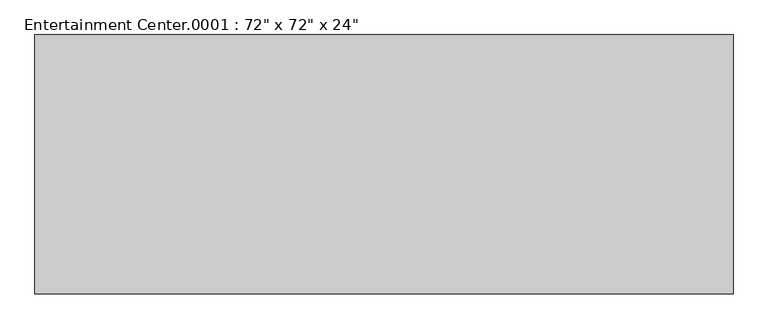
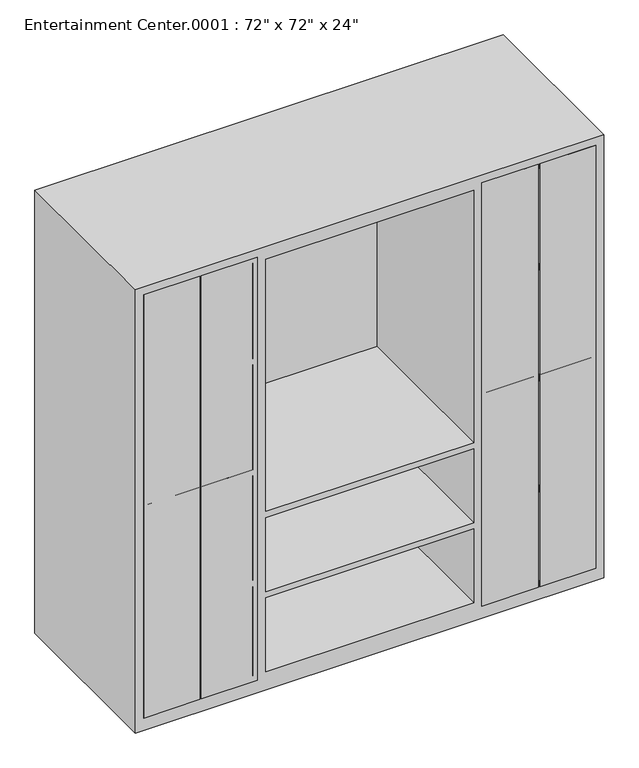
"""IFC4 building model written with IfcOpenShell, lengths in millimetres: furniture geometry."""

from ifc_helpers import new_model, si_unit, point, frame, frame_2d, origin, place, context, project, spatial, polyline, circle_curve, trimmed, segment, composite_curve, outline, extrude, faceted_brep, source, transform, mapped, element, save


def furniture_88072bd9(model_context):
    return source(origin(), model_context, "Body", "SolidModel", [
        extrude(outline(polyline([(-882.65, -711.2), (-663.575, -711.2), (-663.575, -781.05), (-882.65, -781.05), (-882.65, -711.2)])), frame((0.0, 0.0, 50.8), z_axis=(0.0, 0.0, 1.0), x_axis=(1.0, 0.0, 0.0)), (0.0, 0.0, 1.0), 1746.25),
        extrude(outline(polyline([(-657.225, -711.2), (-438.15, -711.2), (-438.15, -781.05), (-657.225, -781.05), (-657.225, -711.2)])), frame((0.0, 0.0, 50.8), z_axis=(0.0, 0.0, 1.0), x_axis=(1.0, 0.0, 0.0)), (0.0, 0.0, 1.0), 1746.25),
        extrude(outline(polyline([(663.575, -711.2), (882.65, -711.2), (882.65, -781.05), (663.575, -781.05), (663.575, -711.2)])), frame((0.0, 0.0, 50.8), z_axis=(0.0, 0.0, 1.0), x_axis=(1.0, 0.0, 0.0)), (0.0, 0.0, 1.0), 1746.25),
        extrude(outline(polyline([(438.15, -711.2), (657.225, -711.2), (657.225, -781.05), (438.15, -781.05), (438.15, -711.2)])), frame((0.0, 0.0, 50.8), z_axis=(0.0, 0.0, 1.0), x_axis=(1.0, 0.0, 0.0)), (0.0, 0.0, 1.0), 1746.25),
        extrude(outline(composite_curve([segment(polyline([(1003.3, -632.9986452), (1003.3, -657.225), (825.5, -657.225), (825.5, -632.9986452)]), True, "CONTINUOUS"), segment(trimmed(circle_curve(frame_2d((850.9, -632.9986452)), 25.4), [point((825.5, -632.9986452))], [point((850.9, -607.5986452))], False, "CARTESIAN"), True, "CONTINUOUS"), segment(polyline([(850.9, -607.5986452), (977.9, -607.5986452)]), True, "CONTINUOUS"), segment(trimmed(circle_curve(frame_2d((977.9, -632.9986452)), 25.4), [point((977.9, -607.5986452))], [point((1003.3, -632.9986452))], False, "CARTESIAN"), True, "CONTINUOUS")], self_intersect=False)), frame((0.0, -714.375, 0.0), z_axis=(0.0, 1.0, 0.0), x_axis=(0.0, 0.0, 1.0)), (0.0, 0.0, 1.0), 3.175),
        extrude(outline(composite_curve([segment(trimmed(circle_curve(frame_2d((977.9, -688.18125)), 25.4), [point((1003.3, -688.18125))], [point((977.9, -713.58125))], False, "CARTESIAN"), True, "CONTINUOUS"), segment(polyline([(977.9, -713.58125), (850.9, -713.58125)]), True, "CONTINUOUS"), segment(trimmed(circle_curve(frame_2d((850.9, -688.18125)), 25.4), [point((850.9, -713.58125))], [point((825.5, -688.18125))], False, "CARTESIAN"), True, "CONTINUOUS"), segment(polyline([(825.5, -688.18125), (825.5, -663.575), (1003.3, -663.575), (1003.3, -688.18125)]), True, "CONTINUOUS")], self_intersect=False)), frame((0.0, -714.375, 0.0), z_axis=(0.0, 1.0, 0.0), x_axis=(0.0, 0.0, 1.0)), (0.0, 0.0, 1.0), 3.175),
        extrude(outline(composite_curve([segment(trimmed(circle_curve(frame_2d((977.9, 632.9986452)), 25.4), [point((1003.3, 632.9986452))], [point((977.9, 607.5986452))], False, "CARTESIAN"), True, "CONTINUOUS"), segment(polyline([(977.9, 607.5986452), (850.9, 607.5986452)]), True, "CONTINUOUS"), segment(trimmed(circle_curve(frame_2d((850.9, 632.9986452)), 25.4), [point((850.9, 607.5986452))], [point((825.5, 632.9986452))], False, "CARTESIAN"), True, "CONTINUOUS"), segment(polyline([(825.5, 632.9986452), (825.5, 657.225), (1003.3, 657.225), (1003.3, 632.9986452)]), True, "CONTINUOUS")], self_intersect=False)), frame((0.0, -714.375, 0.0), z_axis=(0.0, 1.0, 0.0), x_axis=(0.0, 0.0, 1.0)), (0.0, 0.0, 1.0), 3.175),
        extrude(outline(composite_curve([segment(polyline([(1003.3, 688.18125), (1003.3, 663.575), (825.5, 663.575), (825.5, 688.18125)]), True, "CONTINUOUS"), segment(trimmed(circle_curve(frame_2d((850.9, 688.18125)), 25.4), [point((825.5, 688.18125))], [point((850.9, 713.58125))], False, "CARTESIAN"), True, "CONTINUOUS"), segment(polyline([(850.9, 713.58125), (977.9, 713.58125)]), True, "CONTINUOUS"), segment(trimmed(circle_curve(frame_2d((977.9, 688.18125)), 25.4), [point((977.9, 713.58125))], [point((1003.3, 688.18125))], False, "CARTESIAN"), True, "CONTINUOUS")], self_intersect=False)), frame((0.0, -714.375, 0.0), z_axis=(0.0, 1.0, 0.0), x_axis=(0.0, 0.0, 1.0)), (0.0, 0.0, 1.0), 3.175),
        faceted_brep([(914.4, -781.05, 0.0), (914.4, -781.05, 1828.8), (-914.4, -781.05, 1828.8), (-914.4, -781.05, 0.0), (-457.2, -781.05, 1778.0), (-457.2, -781.05, 1384.3), (-863.6, -781.05, 1384.3), (-863.6, -781.05, 1778.0), (-457.2, -781.05, 76.2), (-863.6, -781.05, 76.2), (-863.6, -781.05, 444.5), (-457.2, -781.05, 444.5), (863.6, -781.05, 1384.3), (457.2, -781.05, 1384.3), (457.2, -781.05, 1778.0), (863.6, -781.05, 1778.0), (-406.4, -781.05, 736.6), (-406.4, -781.05, 1778.0), (406.4, -781.05, 1778.0), (406.4, -781.05, 736.6), (406.4, -781.05, 76.2), (-406.4, -781.05, 76.2), (-406.4, -781.05, 381.0), (406.4, -781.05, 381.0), (863.6, -781.05, 76.2), (457.2, -781.05, 76.2), (457.2, -781.05, 444.5), (863.6, -781.05, 444.5), (-863.6, -781.05, 469.9), (-863.6, -781.05, 901.7), (-457.2, -781.05, 901.7), (-457.2, -781.05, 469.9), (-457.2, -781.05, 1358.9), (-457.2, -781.05, 927.1), (-863.6, -781.05, 927.1), (-863.6, -781.05, 1358.9), (457.2, -781.05, 1358.9), (863.6, -781.05, 1358.9), (863.6, -781.05, 927.1), (457.2, -781.05, 927.1), (457.2, -781.05, 901.7), (863.6, -781.05, 901.7), (863.6, -781.05, 469.9), (457.2, -781.05, 469.9), (406.4, -781.05, 406.4), (-406.4, -781.05, 406.4), (-406.4, -781.05, 711.2), (406.4, -781.05, 711.2), (914.4, -101.6, 0.0), (-914.4, -101.6, 0.0), (-914.4, -101.6, 1828.8), (914.4, -101.6, 1828.8), (-457.2, -127.0, 1778.0), (-457.2, -127.0, 1384.3), (-863.6, -127.0, 1384.3), (-863.6, -127.0, 1778.0), (-457.2, -127.0, 76.2), (-863.6, -127.0, 76.2), (-863.6, -127.0, 444.5), (-457.2, -127.0, 444.5), (863.6, -127.0, 1384.3), (457.2, -127.0, 1384.3), (457.2, -127.0, 1778.0), (863.6, -127.0, 1778.0), (-406.4, -127.0, 736.6), (-406.4, -127.0, 1778.0), (406.4, -127.0, 1778.0), (406.4, -127.0, 736.6), (406.4, -127.0, 76.2), (-406.4, -127.0, 76.2), (-406.4, -127.0, 381.0), (406.4, -127.0, 381.0), (863.6, -127.0, 76.2), (457.2, -127.0, 76.2), (457.2, -127.0, 444.5), (863.6, -127.0, 444.5), (-863.6, -127.0, 469.9), (-863.6, -127.0, 901.7), (-457.2, -127.0, 901.7), (-457.2, -127.0, 469.9), (-457.2, -127.0, 1358.9), (-457.2, -127.0, 927.1), (-863.6, -127.0, 927.1), (-863.6, -127.0, 1358.9), (457.2, -127.0, 1358.9), (863.6, -127.0, 1358.9), (863.6, -127.0, 927.1), (457.2, -127.0, 927.1), (457.2, -127.0, 901.7), (863.6, -127.0, 901.7), (863.6, -127.0, 469.9), (457.2, -127.0, 469.9), (406.4, -127.0, 406.4), (-406.4, -127.0, 406.4), (-406.4, -127.0, 711.2), (406.4, -127.0, 711.2)], [[[0, 1, 2, 3], [4, 5, 6, 7], [8, 9, 10, 11], [12, 13, 14, 15], [16, 17, 18, 19], [20, 21, 22, 23], [24, 25, 26, 27], [28, 29, 30, 31], [32, 33, 34, 35], [36, 37, 38, 39], [40, 41, 42, 43], [44, 45, 46, 47]], [[48, 49, 50, 51]], [[1, 0, 48, 51]], [[2, 1, 51, 50]], [[3, 2, 50, 49]], [[0, 3, 49, 48]], [[5, 4, 52, 53]], [[6, 5, 53, 54]], [[7, 6, 54, 55]], [[4, 7, 55, 52]], [[9, 8, 56, 57]], [[10, 9, 57, 58]], [[11, 10, 58, 59]], [[8, 11, 59, 56]], [[13, 12, 60, 61]], [[14, 13, 61, 62]], [[15, 14, 62, 63]], [[12, 15, 63, 60]], [[17, 16, 64, 65]], [[18, 17, 65, 66]], [[19, 18, 66, 67]], [[16, 19, 67, 64]], [[21, 20, 68, 69]], [[22, 21, 69, 70]], [[23, 22, 70, 71]], [[20, 23, 71, 68]], [[25, 24, 72, 73]], [[26, 25, 73, 74]], [[27, 26, 74, 75]], [[24, 27, 75, 72]], [[29, 28, 76, 77]], [[30, 29, 77, 78]], [[31, 30, 78, 79]], [[28, 31, 79, 76]], [[33, 32, 80, 81]], [[34, 33, 81, 82]], [[35, 34, 82, 83]], [[32, 35, 83, 80]], [[37, 36, 84, 85]], [[38, 37, 85, 86]], [[39, 38, 86, 87]], [[36, 39, 87, 84]], [[41, 40, 88, 89]], [[42, 41, 89, 90]], [[43, 42, 90, 91]], [[40, 43, 91, 88]], [[45, 44, 92, 93]], [[46, 45, 93, 94]], [[47, 46, 94, 95]], [[44, 47, 95, 92]], [[53, 52, 55, 54]], [[57, 56, 59, 58]], [[61, 60, 63, 62]], [[65, 64, 67, 66]], [[69, 68, 71, 70]], [[73, 72, 75, 74]], [[77, 76, 79, 78]], [[81, 80, 83, 82]], [[85, 84, 87, 86]], [[89, 88, 91, 90]], [[93, 92, 95, 94]]]),
    ])


if __name__ == "__main__":
    model = new_model("IFC4")
    model_context = context("Model", 3, world=origin())
    ifc_project = project(units=[si_unit("LENGTHUNIT", "METRE", prefix="MILLI")], contexts=[model_context])
    site = spatial("IfcSite", under=ifc_project)
    building = spatial("IfcBuilding", under=site)
    placement = place(None, origin())
    furniture_shape = furniture_88072bd9(model_context)
    element("IfcFurniture", 1, ObjectType="Entertainment Center.0001 : 72\" x 72\" x 24\"", at=placement, inside=building, context=model_context, shape_type="MappedRepresentation", body=[
        mapped(furniture_shape, transform((0.0, 0.0, 0.0), x_axis=(1.0, 0.0, 0.0), y_axis=(0.0, 1.0, 0.0), z_axis=(0.0, 0.0, 1.0))),
    ])
    save(model, "model.ifc")

# Revit data of these elements
# Type "Entertainment Center.0001 : 72\" x 72\" x 24\""
#   Assembly Code = "E2020200"
#   Center Width = 2' - 8"
#   Depth = 2' - 0"
#   Height = 6' - 0"
#   Width = 6' - 0"
#   Material = none
#   Default Elevation = 0
# Element 1 (IfcFurniture, "Entertainment Center.0001 : 72\" x 72\" x 24\"")
#   Materials on its faces: "Steel, Chrome Plated", "Glass - Clear, Grey"
# Materials
#   "Steel, Chrome Plated": class "Metal", colour RGB 17 17 17, transparency 0, Description = "Chromiuim plated steel", Cost = 0
#   "Glass - Clear, Grey": class "Glass", colour RGB 252 255 255, transparency 0.64
